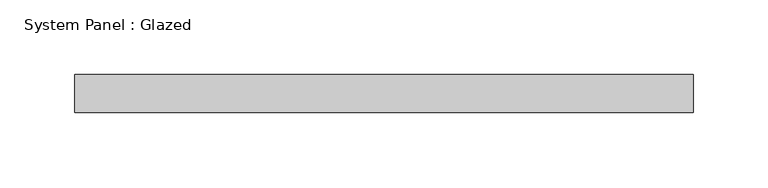
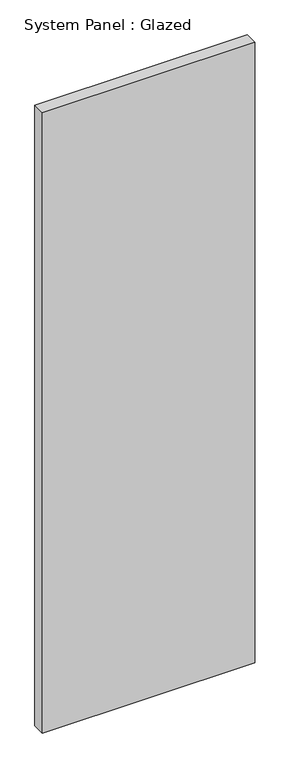
"""IFC4 building model written with IfcOpenShell, lengths in millimetres: plate geometry, System Panel : Glazed."""

from ifc_helpers import new_model, si_unit, origin, origin_with_axes, place, context, project, spatial, polyline, outline, extrude, source, transform, mapped, element, save


def system_panel_glazed_85fa307d(model_context):
    return source(origin(), model_context, "Body", "SweptSolid", [
        extrude(outline(polyline([(206.375, 19.05), (-206.375, 19.05), (-206.375, 44.45), (206.375, 44.45), (206.375, 19.05)])), origin_with_axes(), (0.0, 0.0, 1.0), 1274.633189),
    ])


if __name__ == "__main__":
    model = new_model("IFC4")
    model_context = context("Model", 3, world=origin())
    ifc_project = project(units=[si_unit("LENGTHUNIT", "METRE", prefix="MILLI")], contexts=[model_context])
    site = spatial("IfcSite", under=ifc_project)
    building = spatial("IfcBuilding", under=site)
    placement = place(None, origin())
    system_panel_glazed_shape = system_panel_glazed_85fa307d(model_context)
    element("IfcPlate", 1, ObjectType="System Panel : Glazed", at=placement, inside=building, context=model_context, shape_type="MappedRepresentation", body=[
        mapped(system_panel_glazed_shape, transform((0.0, 0.0, 0.0), x_axis=(1.0, 0.0, 0.0), y_axis=(0.0, 1.0, 0.0), z_axis=(0.0, 0.0, 1.0))),
    ])
    save(model, "model.ifc")

# Revit data of these elements
# Type "System Panel : Glazed"
#   Construction Type Id = "GSP4R"
#   Analytic Construction = "1/8 in Pilkington single glazing"
#   Visual Light Transmittance = 0.9
#   Solar Heat Gain Coefficient = 0.86
#   Heat Transfer Coefficient (U) = 1.18115 BTU/(h·ft²·°F)
#   Define Thermal Properties by = 1
# Element 1 (IfcPlate, "System Panel : Glazed")
#   Materials on its faces: "Glass"
# Materials
#   "Glass": class "Glass", colour RGB 0 128 192, transparency 0.75, Description = "Soda Lime Glass", Cost = 0
